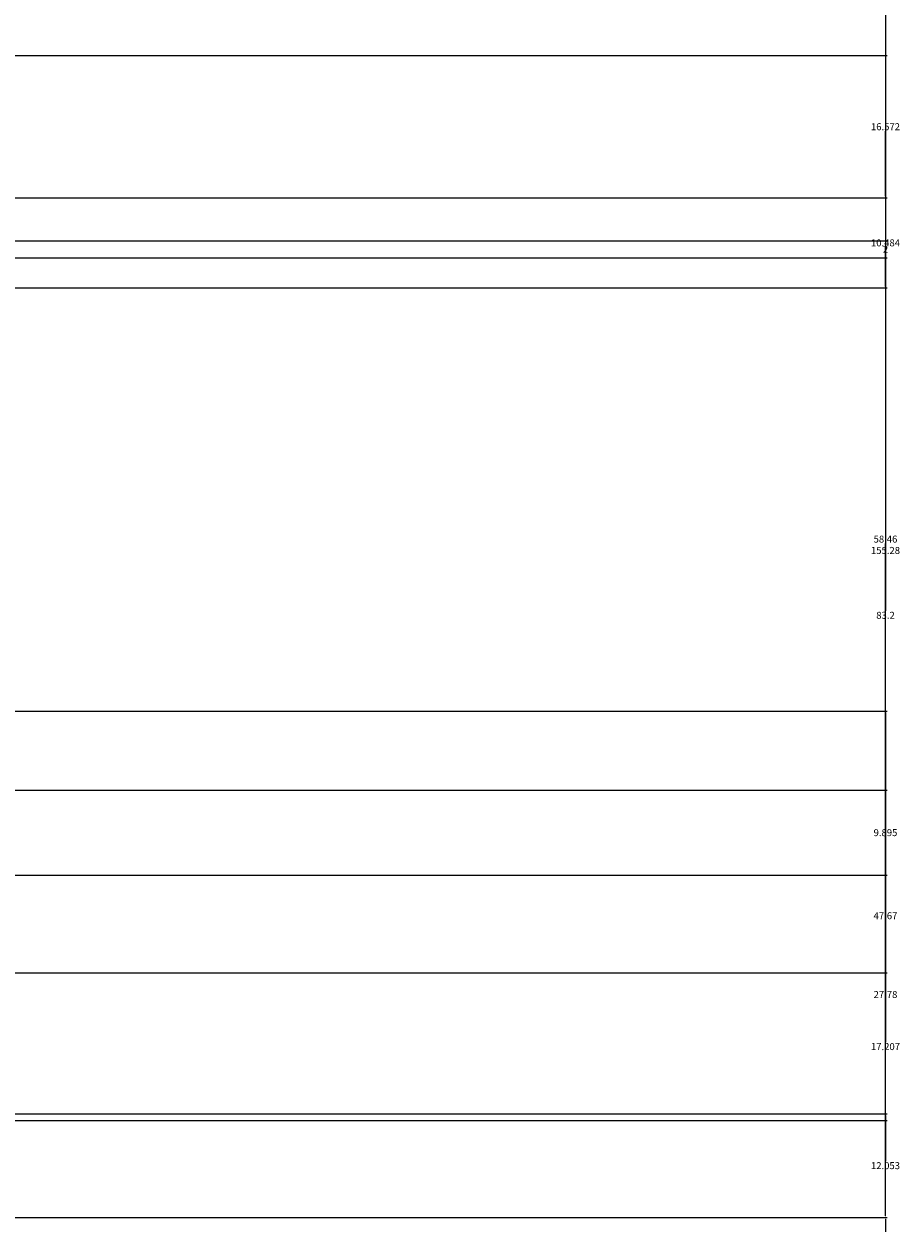
# Model space of a CAD drawing. Units: inches. Extents: x 36 to 594, y 79 to 831.
# Tile 13 of 30: x 492 to 594, y 150 to 290. Entities that reach past the tile are written whole.
import ezdxf

# ---------------------------------------------------------------- set-up
doc = ezdxf.new("R2010")
doc.units = ezdxf.units.IN
doc.header["$MEASUREMENT"] = 0
doc.layers.add('A-ANNO-DIMS', color=2, linetype='Continuous', lineweight=18)
doc.styles.get("Standard").update_dxf_attribs({"font": 'arial.ttf'})
doc.dimstyles.get("Standard").update_dxf_attribs({"dimtxt": 0.8125, "dimasz": 0.18, "dimexe": 0.18, "dimexo": 0.0625, "dimgap": 0.09, "dimtad": 0, "dimtih": 1, "dimtoh": 1, "dimdec": 4, "dimzin": 0, "dimdsep": 46, "dimlunit": 4, "dimtxsty": 'Standard', "dimcen": 0.09, "dimadec": 0, "dimazin": 0, "dimtfac": 1, "dimtdec": 4, "dimtofl": 0, "dimtmove": 0, "dimatfit": 3, "dimfxl": 1, "dimtolj": 1, "dimtzin": 0, "dimarcsym": 0})

# ---------------------------------------------------------------- blocks, each defined once
blk = doc.blocks.new('*D30')
at = {"layer": 'A-ANNO-DIMS', "color": 0, "lineweight": -2, "transparency": 16777216}
for p, q in [((401.61, 150.93), (592.85, 150.93)), ((592.67, 150.75), (592.67, 147.08)), ((592.67, 142.39), (592.67, 146.07)), ((401.61, 142.21), (592.85, 142.21))]:
    blk.add_line(p, q, dxfattribs=at)
at = {"layer": 'A-ANNO-DIMS', "color": 0, "transparency": 16777216}
for points in [[(592.64, 150.75), (592.7, 150.75), (592.67, 150.93)], [(592.64, 142.39), (592.7, 142.39), (592.67, 142.21)]]:
    blk.add_solid(points, dxfattribs=at)
at = {"layer": 'Defpoints', "color": 0, "transparency": 16777216}
for p in [(401.55, 150.93), (592.67, 150.93), (401.55, 142.21)]:
    blk.add_point(p, dxfattribs=at)
at = {"layer": 'A-ANNO-DIMS', "color": 0, "transparency": 16777216, "insert": (592.67, 146.57), "char_height": 0.812, "attachment_point": 5}
blk.add_mtext('\\A1;8.722', dxfattribs=at)
blk = doc.blocks.new('*D31')
at = {"layer": 'A-ANNO-DIMS', "color": 0, "lineweight": -2, "transparency": 16777216}
for p, q in [((448.45, 306.21), (592.85, 306.21)), ((592.67, 306.03), (592.67, 229.08)), ((592.67, 151.11), (592.67, 228.07)), ((401.61, 150.93), (592.85, 150.93))]:
    blk.add_line(p, q, dxfattribs=at)
at = {"layer": 'A-ANNO-DIMS', "color": 0, "transparency": 16777216}
for points in [[(592.64, 306.03), (592.7, 306.03), (592.67, 306.21)], [(592.64, 151.11), (592.7, 151.11), (592.67, 150.93)]]:
    blk.add_solid(points, dxfattribs=at)
at = {"layer": 'Defpoints', "color": 0, "transparency": 16777216}
for p in [(448.39, 306.21), (592.67, 306.21), (401.55, 150.93)]:
    blk.add_point(p, dxfattribs=at)
at = {"layer": 'A-ANNO-DIMS', "color": 0, "transparency": 16777216, "insert": (592.67, 228.57), "char_height": 0.812, "attachment_point": 5}
blk.add_mtext('\\A1;155.28', dxfattribs=at)
blk = doc.blocks.new('*D74')
at = {"layer": 'A-ANNO-DIMS', "color": 0, "lineweight": -2, "transparency": 16777216}
for p, q in [((217.09, 179.42), (592.85, 179.42)), ((592.67, 179.24), (592.67, 171.32)), ((592.67, 162.39), (592.67, 170.31)), ((217.09, 162.21), (592.85, 162.21))]:
    blk.add_line(p, q, dxfattribs=at)
at = {"layer": 'A-ANNO-DIMS', "color": 0, "transparency": 16777216}
for points in [[(592.64, 179.24), (592.7, 179.24), (592.67, 179.42)], [(592.64, 162.39), (592.7, 162.39), (592.67, 162.21)]]:
    blk.add_solid(points, dxfattribs=at)
at = {"layer": 'Defpoints', "color": 0, "transparency": 16777216}
for p in [(217.03, 179.42), (592.67, 179.42), (217.03, 162.21)]:
    blk.add_point(p, dxfattribs=at)
at = {"layer": 'A-ANNO-DIMS', "color": 0, "transparency": 16777216, "insert": (592.67, 170.82), "char_height": 0.812, "attachment_point": 5}
blk.add_mtext('\\A1;17.207', dxfattribs=at)
blk = doc.blocks.new('*D75')
at = {"layer": 'A-ANNO-DIMS', "color": 0, "lineweight": -2, "transparency": 16777216}
for p, q in [((215.09, 262.62), (592.85, 262.62)), ((592.67, 262.44), (592.67, 221.53)), ((592.67, 179.6), (592.67, 220.52)), ((217.09, 179.42), (592.85, 179.42))]:
    blk.add_line(p, q, dxfattribs=at)
at = {"layer": 'A-ANNO-DIMS', "color": 0, "transparency": 16777216}
for points in [[(592.64, 262.44), (592.7, 262.44), (592.67, 262.62)], [(592.64, 179.6), (592.7, 179.6), (592.67, 179.42)]]:
    blk.add_solid(points, dxfattribs=at)
at = {"layer": 'Defpoints', "color": 0, "transparency": 16777216}
for p in [(215.03, 262.62), (592.67, 262.62), (217.03, 179.42)]:
    blk.add_point(p, dxfattribs=at)
at = {"layer": 'A-ANNO-DIMS', "color": 0, "transparency": 16777216, "insert": (592.67, 221.02), "char_height": 0.812, "attachment_point": 5}
blk.add_mtext('\\A1;83.2', dxfattribs=at)
blk = doc.blocks.new('*D76')
at = {"layer": 'A-ANNO-DIMS', "color": 0, "lineweight": -2, "transparency": 16777216}
for p, q in [((217.09, 264.62), (592.85, 264.62)), ((592.67, 264.44), (592.67, 264.12)), ((215.09, 262.62), (592.85, 262.62)), ((592.67, 262.8), (592.67, 263.12))]:
    blk.add_line(p, q, dxfattribs=at)
at = {"layer": 'A-ANNO-DIMS', "color": 0, "transparency": 16777216}
for points in [[(592.64, 264.44), (592.7, 264.44), (592.67, 264.62)], [(592.64, 262.8), (592.7, 262.8), (592.67, 262.62)]]:
    blk.add_solid(points, dxfattribs=at)
at = {"layer": 'Defpoints', "color": 0, "transparency": 16777216}
for p in [(217.03, 264.62), (592.67, 264.62), (215.03, 262.62)]:
    blk.add_point(p, dxfattribs=at)
at = {"layer": 'A-ANNO-DIMS', "color": 0, "transparency": 16777216, "insert": (592.67, 263.62), "char_height": 0.812, "attachment_point": 5}
blk.add_mtext('\\A1;2', dxfattribs=at)
blk = doc.blocks.new('*D77')
at = {"layer": 'A-ANNO-DIMS', "color": 0, "lineweight": -2, "transparency": 16777216}
for p, q in [((151.64, 209.88), (592.85, 209.88)), ((592.67, 209.7), (592.67, 186.55)), ((592.67, 162.39), (592.67, 185.54)), ((156.47, 162.21), (592.85, 162.21))]:
    blk.add_line(p, q, dxfattribs=at)
at = {"layer": 'A-ANNO-DIMS', "color": 0, "transparency": 16777216}
for points in [[(592.64, 209.7), (592.7, 209.7), (592.67, 209.88)], [(592.64, 162.39), (592.7, 162.39), (592.67, 162.21)]]:
    blk.add_solid(points, dxfattribs=at)
at = {"layer": 'Defpoints', "color": 0, "transparency": 16777216}
for p in [(151.58, 209.88), (156.41, 162.21), (592.67, 162.21)]:
    blk.add_point(p, dxfattribs=at)
at = {"layer": 'A-ANNO-DIMS', "color": 0, "transparency": 16777216, "insert": (592.67, 186.05), "char_height": 0.812, "attachment_point": 5}
blk.add_mtext('\\A1;47.67', dxfattribs=at)
blk = doc.blocks.new('*D84')
at = {"layer": 'A-ANNO-DIMS', "color": 0, "lineweight": -2, "transparency": 16777216}
for p, q in [((390.45, 162.99), (592.85, 162.99)), ((592.67, 162.81), (592.67, 157.47)), ((592.67, 151.11), (592.67, 156.46)), ((401.61, 150.93), (592.85, 150.93))]:
    blk.add_line(p, q, dxfattribs=at)
at = {"layer": 'A-ANNO-DIMS', "color": 0, "transparency": 16777216}
for points in [[(592.64, 162.81), (592.7, 162.81), (592.67, 162.99)], [(592.64, 151.11), (592.7, 151.11), (592.67, 150.93)]]:
    blk.add_solid(points, dxfattribs=at)
at = {"layer": 'Defpoints', "color": 0, "transparency": 16777216}
for p in [(390.39, 162.99), (592.67, 162.99), (401.55, 150.93)]:
    blk.add_point(p, dxfattribs=at)
at = {"layer": 'A-ANNO-DIMS', "color": 0, "transparency": 16777216, "insert": (592.67, 156.96), "char_height": 0.812, "attachment_point": 5}
blk.add_mtext('\\A1;12.053', dxfattribs=at)
blk = doc.blocks.new('*D85')
at = {"layer": 'A-ANNO-DIMS', "color": 0, "lineweight": -2, "transparency": 16777216}
for p, q in [((390.45, 190.77), (592.85, 190.77)), ((592.67, 190.59), (592.67, 177.38)), ((592.67, 163.17), (592.67, 176.37)), ((390.45, 162.99), (592.85, 162.99))]:
    blk.add_line(p, q, dxfattribs=at)
at = {"layer": 'A-ANNO-DIMS', "color": 0, "transparency": 16777216}
for points in [[(592.64, 190.59), (592.7, 190.59), (592.67, 190.77)], [(592.64, 163.17), (592.7, 163.17), (592.67, 162.99)]]:
    blk.add_solid(points, dxfattribs=at)
at = {"layer": 'Defpoints', "color": 0, "transparency": 16777216}
for p in [(390.39, 190.77), (592.67, 190.77), (390.39, 162.99)]:
    blk.add_point(p, dxfattribs=at)
at = {"layer": 'A-ANNO-DIMS', "color": 0, "transparency": 16777216, "insert": (592.67, 176.88), "char_height": 0.812, "attachment_point": 5}
blk.add_mtext('\\A1;27.78', dxfattribs=at)
blk = doc.blocks.new('*D86')
at = {"layer": 'A-ANNO-DIMS', "color": 0, "lineweight": -2, "transparency": 16777216}
for p, q in [((390.45, 200.66), (592.85, 200.66)), ((592.67, 200.48), (592.67, 196.22)), ((592.67, 190.95), (592.67, 195.21)), ((390.45, 190.77), (592.85, 190.77))]:
    blk.add_line(p, q, dxfattribs=at)
at = {"layer": 'A-ANNO-DIMS', "color": 0, "transparency": 16777216}
for points in [[(592.64, 200.48), (592.7, 200.48), (592.67, 200.66)], [(592.64, 190.95), (592.7, 190.95), (592.67, 190.77)]]:
    blk.add_solid(points, dxfattribs=at)
at = {"layer": 'Defpoints', "color": 0, "transparency": 16777216}
for p in [(390.39, 200.66), (592.67, 200.66), (390.39, 190.77)]:
    blk.add_point(p, dxfattribs=at)
at = {"layer": 'A-ANNO-DIMS', "color": 0, "transparency": 16777216, "insert": (592.67, 195.72), "char_height": 0.812, "attachment_point": 5}
blk.add_mtext('\\A1;9.895', dxfattribs=at)
blk = doc.blocks.new('*D87')
at = {"layer": 'A-ANNO-DIMS', "color": 0, "lineweight": -2, "transparency": 16777216}
for p, q in [((390.45, 259.12), (592.85, 259.12)), ((592.67, 258.94), (592.67, 230.4)), ((592.67, 200.84), (592.67, 229.39)), ((390.45, 200.66), (592.85, 200.66))]:
    blk.add_line(p, q, dxfattribs=at)
at = {"layer": 'A-ANNO-DIMS', "color": 0, "transparency": 16777216}
for points in [[(592.64, 258.94), (592.7, 258.94), (592.67, 259.12)], [(592.64, 200.84), (592.7, 200.84), (592.67, 200.66)]]:
    blk.add_solid(points, dxfattribs=at)
at = {"layer": 'Defpoints', "color": 0, "transparency": 16777216}
for p in [(390.39, 259.12), (592.67, 259.12), (390.39, 200.66)]:
    blk.add_point(p, dxfattribs=at)
at = {"layer": 'A-ANNO-DIMS', "color": 0, "transparency": 16777216, "insert": (592.67, 229.89), "char_height": 0.812, "attachment_point": 5}
blk.add_mtext('\\A1;58.46', dxfattribs=at)
blk = doc.blocks.new('*D88')
at = {"layer": 'A-ANNO-DIMS', "color": 0, "lineweight": -2, "transparency": 16777216}
for p, q in [((399.61, 269.61), (592.85, 269.61)), ((592.67, 269.43), (592.67, 264.87)), ((592.67, 259.3), (592.67, 263.86)), ((390.45, 259.12), (592.85, 259.12))]:
    blk.add_line(p, q, dxfattribs=at)
at = {"layer": 'A-ANNO-DIMS', "color": 0, "transparency": 16777216}
for points in [[(592.64, 269.43), (592.7, 269.43), (592.67, 269.61)], [(592.64, 259.3), (592.7, 259.3), (592.67, 259.12)]]:
    blk.add_solid(points, dxfattribs=at)
at = {"layer": 'Defpoints', "color": 0, "transparency": 16777216}
for p in [(399.55, 269.61), (592.67, 269.61), (390.39, 259.12)]:
    blk.add_point(p, dxfattribs=at)
at = {"layer": 'A-ANNO-DIMS', "color": 0, "transparency": 16777216, "insert": (592.67, 264.37), "char_height": 0.812, "attachment_point": 5}
blk.add_mtext('\\A1;10.484', dxfattribs=at)
blk = doc.blocks.new('*D89')
at = {"layer": 'A-ANNO-DIMS', "color": 0, "lineweight": -2, "transparency": 16777216}
for p, q in [((401.61, 286.18), (592.85, 286.18)), ((592.67, 286), (592.67, 278.4)), ((592.67, 269.79), (592.67, 277.39)), ((399.61, 269.61), (592.85, 269.61))]:
    blk.add_line(p, q, dxfattribs=at)
at = {"layer": 'A-ANNO-DIMS', "color": 0, "transparency": 16777216}
for points in [[(592.64, 286), (592.7, 286), (592.67, 286.18)], [(592.64, 269.79), (592.7, 269.79), (592.67, 269.61)]]:
    blk.add_solid(points, dxfattribs=at)
at = {"layer": 'Defpoints', "color": 0, "transparency": 16777216}
for p in [(401.55, 286.18), (592.67, 286.18), (399.55, 269.61)]:
    blk.add_point(p, dxfattribs=at)
at = {"layer": 'A-ANNO-DIMS', "color": 0, "transparency": 16777216, "insert": (592.67, 277.89), "char_height": 0.812, "attachment_point": 5}
blk.add_mtext('\\A1;16.572', dxfattribs=at)

msp = doc.modelspace()

# ---------------------------------------------------------------- dimensions: what is measured, and where the dimension line sits
at = {"layer": 'A-ANNO-DIMS'}
for base, p1, p2, override, picture, middle in [((592.6689, 306.2124), (401.5491, 150.9347), (448.3898, 306.2124), {"dimdec": 2, "dimlfac": 1, "dimrnd": 0, "dimzin": 0, "dimdsep": 46, "dimlunit": 2}, '*D31', (592.6689, 228.5735)), ((592.6689, 286.1802), (399.5491, 269.6084), (401.5491, 286.1802), {"dimdec": 3, "dimlfac": 1, "dimrnd": 0, "dimzin": 0, "dimdsep": 46, "dimlunit": 2}, '*D89', (592.6689, 277.8943)), ((592.6689, 269.6084), (390.386, 259.1243), (399.5491, 269.6084), {"dimdec": 3, "dimlfac": 1, "dimrnd": 0, "dimzin": 0, "dimdsep": 46, "dimlunit": 2}, '*D88', (592.6689, 264.3664)), ((592.6689, 264.6224), (215.0273, 262.6224), (217.0273, 264.6224), {"dimdec": 0, "dimlfac": 1, "dimrnd": 0, "dimzin": 0, "dimdsep": 46, "dimlunit": 2}, '*D76', (592.6689, 263.6224)), ((592.6689, 262.6224), (217.0273, 179.4195), (215.0273, 262.6224), {"dimdec": 1, "dimlfac": 1, "dimrnd": 0, "dimzin": 0, "dimdsep": 46, "dimlunit": 2}, '*D75', (592.6689, 221.021)), ((592.6689, 259.1243), (390.386, 200.6645), (390.386, 259.1243), {"dimdec": 2, "dimlfac": 1, "dimrnd": 0, "dimzin": 0, "dimdsep": 46, "dimlunit": 2}, '*D87', (592.6689, 229.8944)), ((592.6689, 162.2124), (151.5799, 209.8823), (156.4069, 162.2124), {"dimdec": 2, "dimlfac": 1, "dimrnd": 0, "dimzin": 0, "dimdsep": 46, "dimlunit": 2}, '*D77', (592.6689, 186.0473)), ((592.6689, 200.6645), (390.386, 190.7697), (390.386, 200.6645), {"dimdec": 3, "dimlfac": 1, "dimrnd": 0, "dimzin": 0, "dimdsep": 46, "dimlunit": 2}, '*D86', (592.6689, 195.7171)), ((592.6689, 190.7697), (390.386, 162.9881), (390.386, 190.7697), {"dimdec": 2, "dimlfac": 1, "dimrnd": 0, "dimzin": 0, "dimdsep": 46, "dimlunit": 2}, '*D85', (592.6689, 176.8789)), ((592.6689, 179.4195), (217.0273, 162.2124), (217.0273, 179.4195), {"dimdec": 3, "dimlfac": 1, "dimrnd": 0, "dimzin": 0, "dimdsep": 46, "dimlunit": 2}, '*D74', (592.6689, 170.8159)), ((592.6689, 162.9881), (401.5491, 150.9347), (390.386, 162.9881), {"dimdec": 3, "dimlfac": 1, "dimrnd": 0, "dimzin": 0, "dimdsep": 46, "dimlunit": 2}, '*D84', (592.6689, 156.9614)), ((592.6689, 150.9347), (401.5491, 142.2124), (401.5491, 150.9347), {"dimdec": 3, "dimlfac": 1, "dimrnd": 0, "dimzin": 0, "dimdsep": 46, "dimlunit": 2}, '*D30', (592.6689, 146.5735))]:
    dim = msp.add_linear_dim(base=base, p1=p1, p2=p2, angle=90, dimstyle='Standard', override=override, dxfattribs=at)
    dim.commit()
    dim.dimension.update_dxf_attribs({"geometry": picture, "text_midpoint": middle})

doc.saveas('drawing.dxf')
